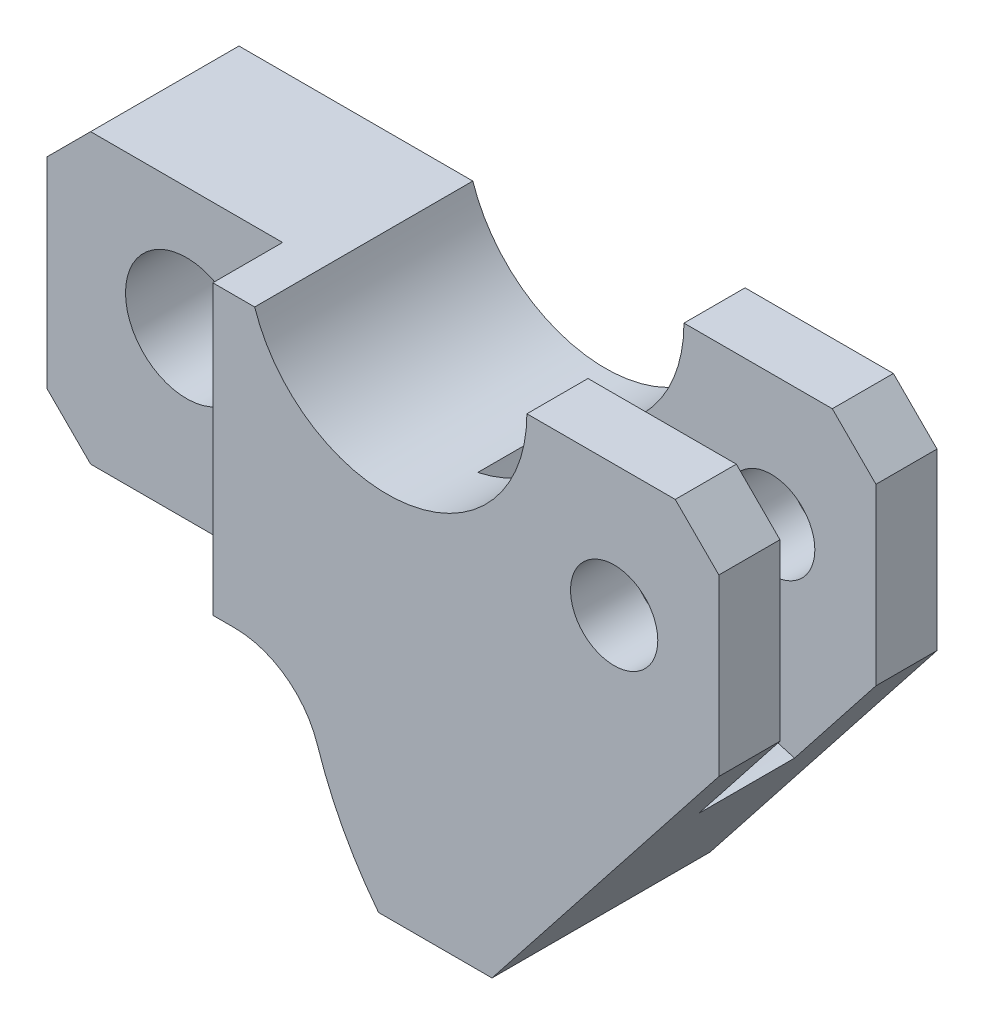
ISO-10303-21;
HEADER;
FILE_DESCRIPTION(('STEP AP214'),'2;1');
FILE_NAME('part.step','',(''),(''),'','','');
FILE_SCHEMA(('AUTOMOTIVE_DESIGN { 1 0 10303 214 1 1 1 1 }'));
ENDSEC;
DATA;
#1=APPLICATION_CONTEXT('core data for automotive mechanical design processes');
#2=APPLICATION_PROTOCOL_DEFINITION('international standard','automotive_design',2000,#1);
#3=PRODUCT_CONTEXT('',#1,'mechanical');
#4=PRODUCT('Part','Part','',(#3));
#5=PRODUCT_RELATED_PRODUCT_CATEGORY('part','',(#4));
#6=PRODUCT_DEFINITION_FORMATION('','',#4);
#7=PRODUCT_DEFINITION_CONTEXT('part definition',#1,'design');
#8=PRODUCT_DEFINITION('design','',#6,#7);
#9=PRODUCT_DEFINITION_SHAPE('','',#8);
#10=(LENGTH_UNIT() NAMED_UNIT(*) SI_UNIT(.MILLI.,.METRE.));
#11=(NAMED_UNIT(*) PLANE_ANGLE_UNIT() SI_UNIT($,.RADIAN.));
#12=(NAMED_UNIT(*) SI_UNIT($,.STERADIAN.) SOLID_ANGLE_UNIT());
#13=UNCERTAINTY_MEASURE_WITH_UNIT(LENGTH_MEASURE(1.E-05),#10,'distance_accuracy_value','');
#14=(GEOMETRIC_REPRESENTATION_CONTEXT(3) GLOBAL_UNCERTAINTY_ASSIGNED_CONTEXT((#13)) GLOBAL_UNIT_ASSIGNED_CONTEXT((#10,
#11,#12)) REPRESENTATION_CONTEXT('',''));
#15=CARTESIAN_POINT('',(0.,0.,0.));
#16=DIRECTION('',(0.,0.,1.));
#17=DIRECTION('',(1.,0.,0.));
#18=AXIS2_PLACEMENT_3D('',#15,#16,#17);
#19=CARTESIAN_POINT('',(0.,-3.84,12.5));
#20=DIRECTION('',(0.,0.,-1.));
#21=DIRECTION('',(-1.,0.,0.));
#22=AXIS2_PLACEMENT_3D('',#19,#20,#21);
#23=CYLINDRICAL_SURFACE('',#22,16.);
#24=CARTESIAN_POINT('',(0.,-3.84,-5.5));
#25=DIRECTION('',(0.,0.,1.));
#26=DIRECTION('',(1.,0.,0.));
#27=AXIS2_PLACEMENT_3D('',#24,#25,#26);
#28=CIRCLE('',#27,16.);
#29=CARTESIAN_POINT('',(16.,-3.84,-5.5));
#30=VERTEX_POINT('',#29);
#31=CARTESIAN_POINT('',(3.3684210526316,-19.4814110492688,-5.5));
#32=VERTEX_POINT('',#31);
#33=EDGE_CURVE('E222',#30,#32,#28,.F.);
#34=ORIENTED_EDGE('',*,*,#33,.F.);
#35=DIRECTION('',(0.,0.,-1.));
#36=VECTOR('',#35,1.);
#37=CARTESIAN_POINT('',(16.,-3.84,12.5));
#38=LINE('',#37,#36);
#39=CARTESIAN_POINT('',(16.,-3.84,-12.5));
#40=VERTEX_POINT('',#39);
#41=EDGE_CURVE('E277',#30,#40,#38,.T.);
#42=ORIENTED_EDGE('',*,*,#41,.T.);
#43=CARTESIAN_POINT('',(0.,-3.84,-12.5));
#44=DIRECTION('',(0.,0.,-1.));
#45=DIRECTION('',(1.,0.,0.));
#46=AXIS2_PLACEMENT_3D('',#43,#44,#45);
#47=CIRCLE('',#46,16.);
#48=CARTESIAN_POINT('',(-15.1986841535706,-8.84,-12.5));
#49=VERTEX_POINT('',#48);
#50=EDGE_CURVE('E251',#40,#49,#47,.T.);
#51=ORIENTED_EDGE('',*,*,#50,.T.);
#52=DIRECTION('',(0.,0.,-1.));
#53=VECTOR('',#52,1.);
#54=CARTESIAN_POINT('',(-15.1986841535706,-8.84,12.5));
#55=LINE('',#54,#53);
#56=CARTESIAN_POINT('',(-15.1986841535706,-8.84,12.5));
#57=VERTEX_POINT('',#56);
#58=EDGE_CURVE('E318',#57,#49,#55,.T.);
#59=ORIENTED_EDGE('',*,*,#58,.F.);
#60=CARTESIAN_POINT('',(0.,-3.84,12.5));
#61=DIRECTION('',(0.,0.,-1.));
#62=DIRECTION('',(1.,0.,0.));
#63=AXIS2_PLACEMENT_3D('',#60,#61,#62);
#64=CIRCLE('',#63,16.);
#65=CARTESIAN_POINT('',(16.,-3.84,12.5));
#66=VERTEX_POINT('',#65);
#67=EDGE_CURVE('E255',#66,#57,#64,.T.);
#68=ORIENTED_EDGE('',*,*,#67,.F.);
#69=CARTESIAN_POINT('',(16.,-3.84,5.5));
#70=VERTEX_POINT('',#69);
#71=EDGE_CURVE('E206',#66,#70,#38,.T.);
#72=ORIENTED_EDGE('',*,*,#71,.T.);
#73=CARTESIAN_POINT('',(0.,-3.84,5.5));
#74=DIRECTION('',(0.,0.,1.));
#75=DIRECTION('',(1.,0.,0.));
#76=AXIS2_PLACEMENT_3D('',#73,#74,#75);
#77=CIRCLE('',#76,16.);
#78=CARTESIAN_POINT('',(3.3684210526316,-19.4814110492688,5.5));
#79=VERTEX_POINT('',#78);
#80=EDGE_CURVE('E200',#70,#79,#77,.F.);
#81=ORIENTED_EDGE('',*,*,#80,.T.);
#82=DIRECTION('',(0.,0.,1.));
#83=VECTOR('',#82,1.);
#84=CARTESIAN_POINT('',(3.3684210526316,-19.4814110492688,0.));
#85=LINE('',#84,#83);
#86=EDGE_CURVE('E188',#79,#32,#85,.F.);
#87=ORIENTED_EDGE('',*,*,#86,.T.);
#88=EDGE_LOOP('',(#34,#42,#51,#59,#68,#72,#81,#87));
#89=FACE_BOUND('',#88,.T.);
#90=ADVANCED_FACE('F41',(#89),#23,.F.);
#91=CARTESIAN_POINT('',(38.,-28.84,12.5));
#92=DIRECTION('',(-0.785491672227536,0.618872226603513,0.));
#93=DIRECTION('',(-0.618872226603513,-0.785491672227536,0.));
#94=AXIS2_PLACEMENT_3D('',#91,#92,#93);
#95=PLANE('',#94);
#96=DIRECTION('',(0.618872226603513,0.785491672227536,0.));
#97=VECTOR('',#96,1.);
#98=CARTESIAN_POINT('',(38.,-28.84,-5.5));
#99=LINE('',#98,#97);
#100=CARTESIAN_POINT('',(28.6733537111755,-40.677666443508,-5.5));
#101=VERTEX_POINT('',#100);
#102=CARTESIAN_POINT('',(38.,-28.84,-5.5));
#103=VERTEX_POINT('',#102);
#104=EDGE_CURVE('E218',#101,#103,#99,.T.);
#105=ORIENTED_EDGE('',*,*,#104,.F.);
#106=DIRECTION('',(0.,0.,1.));
#107=VECTOR('',#106,1.);
#108=CARTESIAN_POINT('',(28.6733537111755,-40.677666443508,-5.5));
#109=LINE('',#108,#107);
#110=CARTESIAN_POINT('',(28.6733537111755,-40.677666443508,5.5));
#111=VERTEX_POINT('',#110);
#112=EDGE_CURVE('E11',#101,#111,#109,.T.);
#113=ORIENTED_EDGE('',*,*,#112,.T.);
#114=DIRECTION('',(0.618872226603513,0.785491672227536,0.));
#115=VECTOR('',#114,1.);
#116=CARTESIAN_POINT('',(38.,-28.84,5.5));
#117=LINE('',#116,#115);
#118=CARTESIAN_POINT('',(38.,-28.84,5.5));
#119=VERTEX_POINT('',#118);
#120=EDGE_CURVE('E203',#111,#119,#117,.T.);
#121=ORIENTED_EDGE('',*,*,#120,.T.);
#122=DIRECTION('',(0.,0.,-1.));
#123=VECTOR('',#122,1.);
#124=CARTESIAN_POINT('',(38.,-28.84,12.5));
#125=LINE('',#124,#123);
#126=CARTESIAN_POINT('',(38.,-28.84,12.5));
#127=VERTEX_POINT('',#126);
#128=EDGE_CURVE('E305',#127,#119,#125,.T.);
#129=ORIENTED_EDGE('',*,*,#128,.F.);
#130=DIRECTION('',(0.618872226603513,0.785491672227535,0.));
#131=VECTOR('',#130,1.);
#132=CARTESIAN_POINT('',(38.,-28.84,12.5));
#133=LINE('',#132,#131);
#134=CARTESIAN_POINT('',(12.,-61.84,12.5));
#135=VERTEX_POINT('',#134);
#136=EDGE_CURVE('E267',#135,#127,#133,.T.);
#137=ORIENTED_EDGE('',*,*,#136,.F.);
#138=DIRECTION('',(0.,0.,-1.));
#139=VECTOR('',#138,1.);
#140=CARTESIAN_POINT('',(12.,-61.84,12.5));
#141=LINE('',#140,#139);
#142=CARTESIAN_POINT('',(12.,-61.84,-12.5));
#143=VERTEX_POINT('',#142);
#144=EDGE_CURVE('E308',#135,#143,#141,.T.);
#145=ORIENTED_EDGE('',*,*,#144,.T.);
#146=DIRECTION('',(0.618872226603513,0.785491672227535,0.));
#147=VECTOR('',#146,1.);
#148=CARTESIAN_POINT('',(38.,-28.84,-12.5));
#149=LINE('',#148,#147);
#150=CARTESIAN_POINT('',(38.,-28.84,-12.5));
#151=VERTEX_POINT('',#150);
#152=EDGE_CURVE('E291',#143,#151,#149,.T.);
#153=ORIENTED_EDGE('',*,*,#152,.T.);
#154=EDGE_CURVE('E301',#103,#151,#125,.T.);
#155=ORIENTED_EDGE('',*,*,#154,.F.);
#156=EDGE_LOOP('',(#105,#113,#121,#129,#137,#145,#153,#155));
#157=FACE_BOUND('',#156,.T.);
#158=ADVANCED_FACE('F392',(#157),#95,.F.);
#159=CARTESIAN_POINT('',(38.,-3.84,12.5));
#160=DIRECTION('',(-1.,0.,0.));
#161=DIRECTION('',(0.,-1.,0.));
#162=AXIS2_PLACEMENT_3D('',#159,#160,#161);
#163=PLANE('',#162);
#164=DIRECTION('',(0.,1.,0.));
#165=VECTOR('',#164,1.);
#166=CARTESIAN_POINT('',(38.,-3.84,-5.5));
#167=LINE('',#166,#165);
#168=CARTESIAN_POINT('',(38.,-8.84000000000001,-5.5));
#169=VERTEX_POINT('',#168);
#170=EDGE_CURVE('E220',#103,#169,#167,.T.);
#171=ORIENTED_EDGE('',*,*,#170,.F.);
#172=ORIENTED_EDGE('',*,*,#154,.T.);
#173=DIRECTION('',(0.,1.,0.));
#174=VECTOR('',#173,1.);
#175=CARTESIAN_POINT('',(38.,-3.84,-12.5));
#176=LINE('',#175,#174);
#177=CARTESIAN_POINT('',(38.,-8.84000000000001,-12.5));
#178=VERTEX_POINT('',#177);
#179=EDGE_CURVE('E298',#151,#178,#176,.T.);
#180=ORIENTED_EDGE('',*,*,#179,.T.);
#181=DIRECTION('',(0.,0.,1.));
#182=VECTOR('',#181,1.);
#183=CARTESIAN_POINT('',(38.,-8.84000000000001,12.5));
#184=LINE('',#183,#182);
#185=EDGE_CURVE('E343',#178,#169,#184,.T.);
#186=ORIENTED_EDGE('',*,*,#185,.T.);
#187=EDGE_LOOP('',(#171,#172,#180,#186));
#188=FACE_BOUND('',#187,.T.);
#189=ADVANCED_FACE('F357',(#188),#163,.F.);
#190=CARTESIAN_POINT('',(16.,-3.84,12.5));
#191=DIRECTION('',(0.,-1.,0.));
#192=DIRECTION('',(1.,0.,0.));
#193=AXIS2_PLACEMENT_3D('',#190,#191,#192);
#194=PLANE('',#193);
#195=DIRECTION('',(-1.,0.,0.));
#196=VECTOR('',#195,1.);
#197=CARTESIAN_POINT('',(16.,-3.84,-5.5));
#198=LINE('',#197,#196);
#199=CARTESIAN_POINT('',(33.,-3.84,-5.5));
#200=VERTEX_POINT('',#199);
#201=EDGE_CURVE('E209',#200,#30,#198,.T.);
#202=ORIENTED_EDGE('',*,*,#201,.F.);
#203=DIRECTION('',(0.,0.,-1.));
#204=VECTOR('',#203,1.);
#205=CARTESIAN_POINT('',(33.,-3.84,12.5));
#206=LINE('',#205,#204);
#207=CARTESIAN_POINT('',(33.,-3.84,-12.5));
#208=VERTEX_POINT('',#207);
#209=EDGE_CURVE('E337',#200,#208,#206,.T.);
#210=ORIENTED_EDGE('',*,*,#209,.T.);
#211=DIRECTION('',(-1.,0.,0.));
#212=VECTOR('',#211,1.);
#213=CARTESIAN_POINT('',(16.,-3.84,-12.5));
#214=LINE('',#213,#212);
#215=EDGE_CURVE('E256',#208,#40,#214,.T.);
#216=ORIENTED_EDGE('',*,*,#215,.T.);
#217=ORIENTED_EDGE('',*,*,#41,.F.);
#218=EDGE_LOOP('',(#202,#210,#216,#217));
#219=FACE_BOUND('',#218,.T.);
#220=ADVANCED_FACE('F373',(#219),#194,.F.);
#221=CARTESIAN_POINT('',(26.,-18.84,12.5));
#222=DIRECTION('',(0.,0.,-1.));
#223=DIRECTION('',(-1.,0.,0.));
#224=AXIS2_PLACEMENT_3D('',#221,#222,#223);
#225=CYLINDRICAL_SURFACE('',#224,5.);
#226=CARTESIAN_POINT('',(26.,-18.84,-12.5));
#227=DIRECTION('',(0.,0.,1.));
#228=DIRECTION('',(1.,0.,0.));
#229=AXIS2_PLACEMENT_3D('',#226,#227,#228);
#230=CIRCLE('',#229,5.);
#231=CARTESIAN_POINT('',(31.,-18.84,-12.5));
#232=VERTEX_POINT('',#231);
#233=EDGE_CURVE('E242',#232,#232,#230,.T.);
#234=ORIENTED_EDGE('',*,*,#233,.F.);
#235=EDGE_LOOP('',(#234));
#236=FACE_BOUND('',#235,.T.);
#237=CARTESIAN_POINT('',(26.,-18.84,-5.5));
#238=DIRECTION('',(0.,0.,1.));
#239=DIRECTION('',(1.,0.,0.));
#240=AXIS2_PLACEMENT_3D('',#237,#238,#239);
#241=CIRCLE('',#240,5.);
#242=CARTESIAN_POINT('',(31.,-18.84,-5.5));
#243=VERTEX_POINT('',#242);
#244=EDGE_CURVE('E198',#243,#243,#241,.T.);
#245=ORIENTED_EDGE('',*,*,#244,.T.);
#246=EDGE_LOOP('',(#245));
#247=FACE_BOUND('',#246,.T.);
#248=ADVANCED_FACE('F448',(#236,#247),#225,.F.);
#249=CARTESIAN_POINT('',(33.,-3.84,12.5));
#250=DIRECTION('',(-0.707106781186548,-0.707106781186546,0.));
#251=DIRECTION('',(0.,0.,-1.));
#252=AXIS2_PLACEMENT_3D('',#249,#250,#251);
#253=PLANE('',#252);
#254=ORIENTED_EDGE('',*,*,#209,.F.);
#255=DIRECTION('',(-0.707106781186547,0.707106781186549,0.));
#256=VECTOR('',#255,1.);
#257=CARTESIAN_POINT('',(33.,-3.84,-5.5));
#258=LINE('',#257,#256);
#259=EDGE_CURVE('E49',#200,#169,#258,.F.);
#260=ORIENTED_EDGE('',*,*,#259,.T.);
#261=ORIENTED_EDGE('',*,*,#185,.F.);
#262=DIRECTION('',(-0.707106781186547,0.707106781186549,0.));
#263=VECTOR('',#262,1.);
#264=CARTESIAN_POINT('',(33.,-3.84,-12.5));
#265=LINE('',#264,#263);
#266=EDGE_CURVE('E326',#208,#178,#265,.F.);
#267=ORIENTED_EDGE('',*,*,#266,.F.);
#268=EDGE_LOOP('',(#254,#260,#261,#267));
#269=FACE_BOUND('',#268,.T.);
#270=ADVANCED_FACE('F352',(#269),#253,.F.);
#271=CARTESIAN_POINT('',(0.,-3.84,12.5));
#272=DIRECTION('',(0.,0.,1.));
#273=DIRECTION('',(1.,0.,0.));
#274=AXIS2_PLACEMENT_3D('',#271,#272,#273);
#275=PLANE('',#274);
#276=DIRECTION('',(0.,1.,0.));
#277=VECTOR('',#276,1.);
#278=CARTESIAN_POINT('',(-20.,-8.84,12.5));
#279=LINE('',#278,#277);
#280=CARTESIAN_POINT('',(-20.,-41.84,12.5));
#281=VERTEX_POINT('',#280);
#282=CARTESIAN_POINT('',(-20.,-8.84,12.5));
#283=VERTEX_POINT('',#282);
#284=EDGE_CURVE('E192',#281,#283,#279,.T.);
#285=ORIENTED_EDGE('',*,*,#284,.F.);
#286=DIRECTION('',(1.,0.,0.));
#287=VECTOR('',#286,1.);
#288=CARTESIAN_POINT('',(-47.,-41.84,12.5));
#289=LINE('',#288,#287);
#290=CARTESIAN_POINT('',(-17.5042005852112,-41.84,12.5));
#291=VERTEX_POINT('',#290);
#292=EDGE_CURVE('E261',#281,#291,#289,.T.);
#293=ORIENTED_EDGE('',*,*,#292,.T.);
#294=CARTESIAN_POINT('',(-17.5042005852112,-51.84,12.5));
#295=DIRECTION('',(0.,0.,-1.));
#296=DIRECTION('',(1.,0.,0.));
#297=AXIS2_PLACEMENT_3D('',#294,#295,#296);
#298=CIRCLE('',#297,10.);
#299=CARTESIAN_POINT('',(-8.00180676846029,-48.7247934656955,12.5));
#300=VERTEX_POINT('',#299);
#301=EDGE_CURVE('E263',#291,#300,#298,.T.);
#302=ORIENTED_EDGE('',*,*,#301,.T.);
#303=CARTESIAN_POINT('',(32.8971117805512,-35.3167427400696,12.5));
#304=DIRECTION('',(0.,0.,1.));
#305=DIRECTION('',(1.,0.,0.));
#306=AXIS2_PLACEMENT_3D('',#303,#304,#305);
#307=CIRCLE('',#306,43.0406477964683);
#308=CARTESIAN_POINT('',(-0.999999999999987,-61.84,12.5));
#309=VERTEX_POINT('',#308);
#310=EDGE_CURVE('E264',#300,#309,#307,.T.);
#311=ORIENTED_EDGE('',*,*,#310,.T.);
#312=DIRECTION('',(1.,0.,0.));
#313=VECTOR('',#312,1.);
#314=CARTESIAN_POINT('',(12.,-61.84,12.5));
#315=LINE('',#314,#313);
#316=EDGE_CURVE('E270',#309,#135,#315,.T.);
#317=ORIENTED_EDGE('',*,*,#316,.T.);
#318=ORIENTED_EDGE('',*,*,#136,.T.);
#319=DIRECTION('',(0.,1.,0.));
#320=VECTOR('',#319,1.);
#321=CARTESIAN_POINT('',(38.,-3.84,12.5));
#322=LINE('',#321,#320);
#323=CARTESIAN_POINT('',(38.,-8.84000000000001,12.5));
#324=VERTEX_POINT('',#323);
#325=EDGE_CURVE('E271',#127,#324,#322,.T.);
#326=ORIENTED_EDGE('',*,*,#325,.T.);
#327=DIRECTION('',(0.707106781186547,-0.707106781186549,0.));
#328=VECTOR('',#327,1.);
#329=CARTESIAN_POINT('',(16.5000000000001,12.66,12.5));
#330=LINE('',#329,#328);
#331=CARTESIAN_POINT('',(33.,-3.84,12.5));
#332=VERTEX_POINT('',#331);
#333=EDGE_CURVE('E333',#324,#332,#330,.F.);
#334=ORIENTED_EDGE('',*,*,#333,.T.);
#335=DIRECTION('',(-1.,0.,0.));
#336=VECTOR('',#335,1.);
#337=CARTESIAN_POINT('',(16.,-3.84,12.5));
#338=LINE('',#337,#336);
#339=EDGE_CURVE('E273',#332,#66,#338,.T.);
#340=ORIENTED_EDGE('',*,*,#339,.T.);
#341=ORIENTED_EDGE('',*,*,#67,.T.);
#342=DIRECTION('',(-1.,0.,0.));
#343=VECTOR('',#342,1.);
#344=CARTESIAN_POINT('',(-15.1986841535706,-8.84,12.5));
#345=LINE('',#344,#343);
#346=EDGE_CURVE('E260',#57,#283,#345,.T.);
#347=ORIENTED_EDGE('',*,*,#346,.T.);
#348=EDGE_LOOP('',(#285,#293,#302,#311,#317,#318,#326,#334,#340,#341,#347));
#349=FACE_BOUND('',#348,.T.);
#350=CARTESIAN_POINT('',(26.,-18.84,12.5));
#351=DIRECTION('',(0.,0.,1.));
#352=DIRECTION('',(1.,0.,0.));
#353=AXIS2_PLACEMENT_3D('',#350,#351,#352);
#354=CIRCLE('',#353,5.);
#355=CARTESIAN_POINT('',(31.,-18.84,12.5));
#356=VERTEX_POINT('',#355);
#357=EDGE_CURVE('E244',#356,#356,#354,.T.);
#358=ORIENTED_EDGE('',*,*,#357,.F.);
#359=EDGE_LOOP('',(#358));
#360=FACE_BOUND('',#359,.T.);
#361=ADVANCED_FACE('F385',(#349,#360),#275,.T.);
#362=CARTESIAN_POINT('',(0.,-3.84,-12.5));
#363=DIRECTION('',(0.,0.,1.));
#364=DIRECTION('',(1.,0.,0.));
#365=AXIS2_PLACEMENT_3D('',#362,#363,#364);
#366=PLANE('',#365);
#367=DIRECTION('',(0.,-1.,0.));
#368=VECTOR('',#367,1.);
#369=CARTESIAN_POINT('',(-47.,-8.84,-12.5));
#370=LINE('',#369,#368);
#371=CARTESIAN_POINT('',(-47.,-13.84,-12.5));
#372=VERTEX_POINT('',#371);
#373=CARTESIAN_POINT('',(-47.,-36.84,-12.5));
#374=VERTEX_POINT('',#373);
#375=EDGE_CURVE('E285',#372,#374,#370,.T.);
#376=ORIENTED_EDGE('',*,*,#375,.F.);
#377=DIRECTION('',(-0.707106781186548,-0.707106781186547,0.));
#378=VECTOR('',#377,1.);
#379=CARTESIAN_POINT('',(-47.,-13.84,-12.5));
#380=LINE('',#379,#378);
#381=CARTESIAN_POINT('',(-42.,-8.84,-12.5));
#382=VERTEX_POINT('',#381);
#383=EDGE_CURVE('E329',#372,#382,#380,.F.);
#384=ORIENTED_EDGE('',*,*,#383,.T.);
#385=DIRECTION('',(-1.,0.,0.));
#386=VECTOR('',#385,1.);
#387=CARTESIAN_POINT('',(-15.1986841535706,-8.84,-12.5));
#388=LINE('',#387,#386);
#389=EDGE_CURVE('E276',#49,#382,#388,.T.);
#390=ORIENTED_EDGE('',*,*,#389,.F.);
#391=ORIENTED_EDGE('',*,*,#50,.F.);
#392=ORIENTED_EDGE('',*,*,#215,.F.);
#393=ORIENTED_EDGE('',*,*,#266,.T.);
#394=ORIENTED_EDGE('',*,*,#179,.F.);
#395=ORIENTED_EDGE('',*,*,#152,.F.);
#396=DIRECTION('',(1.,0.,0.));
#397=VECTOR('',#396,1.);
#398=CARTESIAN_POINT('',(12.,-61.84,-12.5));
#399=LINE('',#398,#397);
#400=CARTESIAN_POINT('',(-0.999999999999987,-61.84,-12.5));
#401=VERTEX_POINT('',#400);
#402=EDGE_CURVE('E292',#401,#143,#399,.T.);
#403=ORIENTED_EDGE('',*,*,#402,.F.);
#404=CARTESIAN_POINT('',(32.8971117805512,-35.3167427400696,-12.5));
#405=DIRECTION('',(0.,0.,1.));
#406=DIRECTION('',(1.,0.,0.));
#407=AXIS2_PLACEMENT_3D('',#404,#405,#406);
#408=CIRCLE('',#407,43.0406477964683);
#409=CARTESIAN_POINT('',(-8.00180676846029,-48.7247934656955,-12.5));
#410=VERTEX_POINT('',#409);
#411=EDGE_CURVE('E288',#410,#401,#408,.T.);
#412=ORIENTED_EDGE('',*,*,#411,.F.);
#413=CARTESIAN_POINT('',(-17.5042005852112,-51.84,-12.5));
#414=DIRECTION('',(0.,0.,-1.));
#415=DIRECTION('',(1.,0.,0.));
#416=AXIS2_PLACEMENT_3D('',#413,#414,#415);
#417=CIRCLE('',#416,10.);
#418=CARTESIAN_POINT('',(-17.5042005852112,-41.84,-12.5));
#419=VERTEX_POINT('',#418);
#420=EDGE_CURVE('E286',#419,#410,#417,.T.);
#421=ORIENTED_EDGE('',*,*,#420,.F.);
#422=DIRECTION('',(1.,0.,0.));
#423=VECTOR('',#422,1.);
#424=CARTESIAN_POINT('',(-47.,-41.84,-12.5));
#425=LINE('',#424,#423);
#426=CARTESIAN_POINT('',(-42.,-41.84,-12.5));
#427=VERTEX_POINT('',#426);
#428=EDGE_CURVE('E284',#427,#419,#425,.T.);
#429=ORIENTED_EDGE('',*,*,#428,.F.);
#430=DIRECTION('',(0.707106781186546,-0.707106781186549,0.));
#431=VECTOR('',#430,1.);
#432=CARTESIAN_POINT('',(-42.,-41.84,-12.5));
#433=LINE('',#432,#431);
#434=EDGE_CURVE('E327',#427,#374,#433,.F.);
#435=ORIENTED_EDGE('',*,*,#434,.T.);
#436=EDGE_LOOP('',(#376,#384,#390,#391,#392,#393,#394,#395,#403,#412,#421,#429,#435));
#437=FACE_BOUND('',#436,.T.);
#438=CARTESIAN_POINT('',(-31.,-22.84,-12.5));
#439=DIRECTION('',(0.,0.,1.));
#440=DIRECTION('',(1.,0.,0.));
#441=AXIS2_PLACEMENT_3D('',#438,#439,#440);
#442=CIRCLE('',#441,7.);
#443=CARTESIAN_POINT('',(-24.,-22.84,-12.5));
#444=VERTEX_POINT('',#443);
#445=EDGE_CURVE('E250',#444,#444,#442,.T.);
#446=ORIENTED_EDGE('',*,*,#445,.T.);
#447=EDGE_LOOP('',(#446));
#448=FACE_BOUND('',#447,.T.);
#449=ORIENTED_EDGE('',*,*,#233,.T.);
#450=EDGE_LOOP('',(#449));
#451=FACE_BOUND('',#450,.T.);
#452=ADVANCED_FACE('F368',(#437,#448,#451),#366,.F.);
#453=CARTESIAN_POINT('',(-15.1986841535706,-8.84,12.5));
#454=DIRECTION('',(0.,-1.,0.));
#455=DIRECTION('',(1.,0.,0.));
#456=AXIS2_PLACEMENT_3D('',#453,#454,#455);
#457=PLANE('',#456);
#458=DIRECTION('',(-1.,0.,0.));
#459=VECTOR('',#458,1.);
#460=CARTESIAN_POINT('',(-47.,-8.84,4.5));
#461=LINE('',#460,#459);
#462=CARTESIAN_POINT('',(-20.,-8.84,4.5));
#463=VERTEX_POINT('',#462);
#464=CARTESIAN_POINT('',(-42.,-8.84,4.5));
#465=VERTEX_POINT('',#464);
#466=EDGE_CURVE('E229',#463,#465,#461,.T.);
#467=ORIENTED_EDGE('',*,*,#466,.F.);
#468=DIRECTION('',(0.,0.,1.));
#469=VECTOR('',#468,1.);
#470=CARTESIAN_POINT('',(-20.,-8.84,4.5));
#471=LINE('',#470,#469);
#472=EDGE_CURVE('E232',#463,#283,#471,.T.);
#473=ORIENTED_EDGE('',*,*,#472,.T.);
#474=ORIENTED_EDGE('',*,*,#346,.F.);
#475=ORIENTED_EDGE('',*,*,#58,.T.);
#476=ORIENTED_EDGE('',*,*,#389,.T.);
#477=DIRECTION('',(0.,0.,1.));
#478=VECTOR('',#477,1.);
#479=CARTESIAN_POINT('',(-42.,-8.84,12.5));
#480=LINE('',#479,#478);
#481=EDGE_CURVE('E335',#382,#465,#480,.T.);
#482=ORIENTED_EDGE('',*,*,#481,.T.);
#483=EDGE_LOOP('',(#467,#473,#474,#475,#476,#482));
#484=FACE_BOUND('',#483,.T.);
#485=ADVANCED_FACE('F378',(#484),#457,.F.);
#486=CARTESIAN_POINT('',(-47.,-8.84,12.5));
#487=DIRECTION('',(1.,0.,0.));
#488=DIRECTION('',(0.,0.,-1.));
#489=AXIS2_PLACEMENT_3D('',#486,#487,#488);
#490=PLANE('',#489);
#491=DIRECTION('',(0.,0.,1.));
#492=VECTOR('',#491,1.);
#493=CARTESIAN_POINT('',(-47.,-36.84,12.5));
#494=LINE('',#493,#492);
#495=CARTESIAN_POINT('',(-47.,-36.84,4.5));
#496=VERTEX_POINT('',#495);
#497=EDGE_CURVE('E321',#374,#496,#494,.T.);
#498=ORIENTED_EDGE('',*,*,#497,.T.);
#499=DIRECTION('',(0.,-1.,0.));
#500=VECTOR('',#499,1.);
#501=CARTESIAN_POINT('',(-47.,-8.84,4.5));
#502=LINE('',#501,#500);
#503=CARTESIAN_POINT('',(-47.,-13.84,4.5));
#504=VERTEX_POINT('',#503);
#505=EDGE_CURVE('E64',#504,#496,#502,.T.);
#506=ORIENTED_EDGE('',*,*,#505,.F.);
#507=DIRECTION('',(0.,0.,-1.));
#508=VECTOR('',#507,1.);
#509=CARTESIAN_POINT('',(-47.,-13.84,12.5));
#510=LINE('',#509,#508);
#511=EDGE_CURVE('E322',#504,#372,#510,.T.);
#512=ORIENTED_EDGE('',*,*,#511,.T.);
#513=ORIENTED_EDGE('',*,*,#375,.T.);
#514=EDGE_LOOP('',(#498,#506,#512,#513));
#515=FACE_BOUND('',#514,.T.);
#516=ADVANCED_FACE('F421',(#515),#490,.F.);
#517=CARTESIAN_POINT('',(-47.,-41.84,12.5));
#518=DIRECTION('',(0.,1.,0.));
#519=DIRECTION('',(0.,0.,1.));
#520=AXIS2_PLACEMENT_3D('',#517,#518,#519);
#521=PLANE('',#520);
#522=ORIENTED_EDGE('',*,*,#292,.F.);
#523=DIRECTION('',(0.,0.,1.));
#524=VECTOR('',#523,1.);
#525=CARTESIAN_POINT('',(-20.,-41.84,4.5));
#526=LINE('',#525,#524);
#527=CARTESIAN_POINT('',(-20.,-41.84,4.5));
#528=VERTEX_POINT('',#527);
#529=EDGE_CURVE('E235',#528,#281,#526,.T.);
#530=ORIENTED_EDGE('',*,*,#529,.F.);
#531=DIRECTION('',(1.,0.,0.));
#532=VECTOR('',#531,1.);
#533=CARTESIAN_POINT('',(-47.,-41.84,4.5));
#534=LINE('',#533,#532);
#535=CARTESIAN_POINT('',(-42.,-41.84,4.5));
#536=VERTEX_POINT('',#535);
#537=EDGE_CURVE('E223',#536,#528,#534,.T.);
#538=ORIENTED_EDGE('',*,*,#537,.F.);
#539=DIRECTION('',(0.,0.,-1.));
#540=VECTOR('',#539,1.);
#541=CARTESIAN_POINT('',(-42.,-41.84,12.5));
#542=LINE('',#541,#540);
#543=EDGE_CURVE('E340',#536,#427,#542,.T.);
#544=ORIENTED_EDGE('',*,*,#543,.T.);
#545=ORIENTED_EDGE('',*,*,#428,.T.);
#546=DIRECTION('',(0.,0.,-1.));
#547=VECTOR('',#546,1.);
#548=CARTESIAN_POINT('',(-17.5042005852112,-41.84,12.5));
#549=LINE('',#548,#547);
#550=EDGE_CURVE('E312',#291,#419,#549,.T.);
#551=ORIENTED_EDGE('',*,*,#550,.F.);
#552=EDGE_LOOP('',(#522,#530,#538,#544,#545,#551));
#553=FACE_BOUND('',#552,.T.);
#554=ADVANCED_FACE('F412',(#553),#521,.F.);
#555=CARTESIAN_POINT('',(-17.5042005852112,-51.84,12.5));
#556=DIRECTION('',(0.,0.,-1.));
#557=DIRECTION('',(-1.,0.,0.));
#558=AXIS2_PLACEMENT_3D('',#555,#556,#557);
#559=CYLINDRICAL_SURFACE('',#558,10.);
#560=ORIENTED_EDGE('',*,*,#420,.T.);
#561=DIRECTION('',(0.,0.,-1.));
#562=VECTOR('',#561,1.);
#563=CARTESIAN_POINT('',(-8.00180676846029,-48.7247934656955,12.5));
#564=LINE('',#563,#562);
#565=EDGE_CURVE('E315',#300,#410,#564,.T.);
#566=ORIENTED_EDGE('',*,*,#565,.F.);
#567=ORIENTED_EDGE('',*,*,#301,.F.);
#568=ORIENTED_EDGE('',*,*,#550,.T.);
#569=EDGE_LOOP('',(#560,#566,#567,#568));
#570=FACE_BOUND('',#569,.T.);
#571=ADVANCED_FACE('F414',(#570),#559,.F.);
#572=CARTESIAN_POINT('',(32.8971117805512,-35.3167427400696,12.5));
#573=DIRECTION('',(0.,0.,-1.));
#574=DIRECTION('',(-1.,0.,0.));
#575=AXIS2_PLACEMENT_3D('',#572,#573,#574);
#576=CYLINDRICAL_SURFACE('',#575,43.0406477964683);
#577=ORIENTED_EDGE('',*,*,#411,.T.);
#578=DIRECTION('',(0.,0.,-1.));
#579=VECTOR('',#578,1.);
#580=CARTESIAN_POINT('',(-0.999999999999987,-61.84,12.5));
#581=LINE('',#580,#579);
#582=EDGE_CURVE('E310',#309,#401,#581,.T.);
#583=ORIENTED_EDGE('',*,*,#582,.F.);
#584=ORIENTED_EDGE('',*,*,#310,.F.);
#585=ORIENTED_EDGE('',*,*,#565,.T.);
#586=EDGE_LOOP('',(#577,#583,#584,#585));
#587=FACE_BOUND('',#586,.T.);
#588=ADVANCED_FACE('F408',(#587),#576,.T.);
#589=CARTESIAN_POINT('',(12.,-61.84,12.5));
#590=DIRECTION('',(0.,1.,0.));
#591=DIRECTION('',(-1.,0.,0.));
#592=AXIS2_PLACEMENT_3D('',#589,#590,#591);
#593=PLANE('',#592);
#594=ORIENTED_EDGE('',*,*,#402,.T.);
#595=ORIENTED_EDGE('',*,*,#144,.F.);
#596=ORIENTED_EDGE('',*,*,#316,.F.);
#597=ORIENTED_EDGE('',*,*,#582,.T.);
#598=EDGE_LOOP('',(#594,#595,#596,#597));
#599=FACE_BOUND('',#598,.T.);
#600=ADVANCED_FACE('F397',(#599),#593,.F.);
#601=ORIENTED_EDGE('',*,*,#128,.T.);
#602=DIRECTION('',(0.,1.,0.));
#603=VECTOR('',#602,1.);
#604=CARTESIAN_POINT('',(38.,-3.84,5.5));
#605=LINE('',#604,#603);
#606=CARTESIAN_POINT('',(38.,-8.84000000000001,5.5));
#607=VERTEX_POINT('',#606);
#608=EDGE_CURVE('E215',#119,#607,#605,.T.);
#609=ORIENTED_EDGE('',*,*,#608,.T.);
#610=EDGE_CURVE('E345',#607,#324,#184,.T.);
#611=ORIENTED_EDGE('',*,*,#610,.T.);
#612=ORIENTED_EDGE('',*,*,#325,.F.);
#613=EDGE_LOOP('',(#601,#609,#611,#612));
#614=FACE_BOUND('',#613,.T.);
#615=ADVANCED_FACE('F433',(#614),#163,.F.);
#616=CARTESIAN_POINT('',(33.,-3.84,5.5));
#617=VERTEX_POINT('',#616);
#618=EDGE_CURVE('E339',#332,#617,#206,.T.);
#619=ORIENTED_EDGE('',*,*,#618,.T.);
#620=DIRECTION('',(-1.,0.,0.));
#621=VECTOR('',#620,1.);
#622=CARTESIAN_POINT('',(16.,-3.84,5.5));
#623=LINE('',#622,#621);
#624=EDGE_CURVE('E60',#617,#70,#623,.T.);
#625=ORIENTED_EDGE('',*,*,#624,.T.);
#626=ORIENTED_EDGE('',*,*,#71,.F.);
#627=ORIENTED_EDGE('',*,*,#339,.F.);
#628=EDGE_LOOP('',(#619,#625,#626,#627));
#629=FACE_BOUND('',#628,.T.);
#630=ADVANCED_FACE('F389',(#629),#194,.F.);
#631=CARTESIAN_POINT('',(-31.,-22.84,12.5));
#632=DIRECTION('',(0.,0.,-1.));
#633=DIRECTION('',(-1.,0.,0.));
#634=AXIS2_PLACEMENT_3D('',#631,#632,#633);
#635=CYLINDRICAL_SURFACE('',#634,7.);
#636=CARTESIAN_POINT('',(-31.,-22.84,4.5));
#637=DIRECTION('',(0.,0.,-1.));
#638=DIRECTION('',(-1.,0.,0.));
#639=AXIS2_PLACEMENT_3D('',#636,#637,#638);
#640=CIRCLE('',#639,7.);
#641=CARTESIAN_POINT('',(-38.,-22.84,4.5));
#642=VERTEX_POINT('',#641);
#643=EDGE_CURVE('E243',#642,#642,#640,.T.);
#644=ORIENTED_EDGE('',*,*,#643,.F.);
#645=EDGE_LOOP('',(#644));
#646=FACE_BOUND('',#645,.T.);
#647=ORIENTED_EDGE('',*,*,#445,.F.);
#648=EDGE_LOOP('',(#647));
#649=FACE_BOUND('',#648,.T.);
#650=ADVANCED_FACE('F473',(#646,#649),#635,.F.);
#651=CARTESIAN_POINT('',(26.,-18.84,5.5));
#652=DIRECTION('',(0.,0.,1.));
#653=DIRECTION('',(1.,0.,0.));
#654=AXIS2_PLACEMENT_3D('',#651,#652,#653);
#655=CIRCLE('',#654,5.);
#656=CARTESIAN_POINT('',(31.,-18.84,5.5));
#657=VERTEX_POINT('',#656);
#658=EDGE_CURVE('E210',#657,#657,#655,.T.);
#659=ORIENTED_EDGE('',*,*,#658,.F.);
#660=EDGE_LOOP('',(#659));
#661=FACE_BOUND('',#660,.T.);
#662=ORIENTED_EDGE('',*,*,#357,.T.);
#663=EDGE_LOOP('',(#662));
#664=FACE_BOUND('',#663,.T.);
#665=ADVANCED_FACE('F465',(#661,#664),#225,.F.);
#666=CARTESIAN_POINT('',(-47.,-13.84,12.5));
#667=DIRECTION('',(0.707106781186547,-0.707106781186548,0.));
#668=DIRECTION('',(0.,0.,-1.));
#669=AXIS2_PLACEMENT_3D('',#666,#667,#668);
#670=PLANE('',#669);
#671=DIRECTION('',(0.707106781186548,0.707106781186547,0.));
#672=VECTOR('',#671,1.);
#673=CARTESIAN_POINT('',(-47.,-13.84,4.5));
#674=LINE('',#673,#672);
#675=EDGE_CURVE('E236',#465,#504,#674,.F.);
#676=ORIENTED_EDGE('',*,*,#675,.F.);
#677=ORIENTED_EDGE('',*,*,#481,.F.);
#678=ORIENTED_EDGE('',*,*,#383,.F.);
#679=ORIENTED_EDGE('',*,*,#511,.F.);
#680=EDGE_LOOP('',(#676,#677,#678,#679));
#681=FACE_BOUND('',#680,.T.);
#682=ADVANCED_FACE('F441',(#681),#670,.F.);
#683=CARTESIAN_POINT('',(-42.,-41.84,12.5));
#684=DIRECTION('',(0.707106781186549,0.707106781186546,0.));
#685=DIRECTION('',(0.,0.,-1.));
#686=AXIS2_PLACEMENT_3D('',#683,#684,#685);
#687=PLANE('',#686);
#688=DIRECTION('',(-0.707106781186546,0.707106781186549,0.));
#689=VECTOR('',#688,1.);
#690=CARTESIAN_POINT('',(-42.,-41.84,4.5));
#691=LINE('',#690,#689);
#692=EDGE_CURVE('E350',#496,#536,#691,.F.);
#693=ORIENTED_EDGE('',*,*,#692,.F.);
#694=ORIENTED_EDGE('',*,*,#497,.F.);
#695=ORIENTED_EDGE('',*,*,#434,.F.);
#696=ORIENTED_EDGE('',*,*,#543,.F.);
#697=EDGE_LOOP('',(#693,#694,#695,#696));
#698=FACE_BOUND('',#697,.T.);
#699=ADVANCED_FACE('F426',(#698),#687,.F.);
#700=DIRECTION('',(-0.707106781186547,0.707106781186549,0.));
#701=VECTOR('',#700,1.);
#702=CARTESIAN_POINT('',(33.,-3.84,5.5));
#703=LINE('',#702,#701);
#704=EDGE_CURVE('E349',#617,#607,#703,.F.);
#705=ORIENTED_EDGE('',*,*,#704,.F.);
#706=ORIENTED_EDGE('',*,*,#618,.F.);
#707=ORIENTED_EDGE('',*,*,#333,.F.);
#708=ORIENTED_EDGE('',*,*,#610,.F.);
#709=EDGE_LOOP('',(#705,#706,#707,#708));
#710=FACE_BOUND('',#709,.T.);
#711=ADVANCED_FACE('F42',(#710),#253,.F.);
#712=CARTESIAN_POINT('',(-20.,-8.84,4.5));
#713=DIRECTION('',(1.,0.,0.));
#714=DIRECTION('',(0.,1.,0.));
#715=AXIS2_PLACEMENT_3D('',#712,#713,#714);
#716=PLANE('',#715);
#717=ORIENTED_EDGE('',*,*,#284,.T.);
#718=ORIENTED_EDGE('',*,*,#472,.F.);
#719=DIRECTION('',(0.,1.,0.));
#720=VECTOR('',#719,1.);
#721=CARTESIAN_POINT('',(-20.,-8.84,4.5));
#722=LINE('',#721,#720);
#723=EDGE_CURVE('E230',#528,#463,#722,.T.);
#724=ORIENTED_EDGE('',*,*,#723,.F.);
#725=ORIENTED_EDGE('',*,*,#529,.T.);
#726=EDGE_LOOP('',(#717,#718,#724,#725));
#727=FACE_BOUND('',#726,.T.);
#728=ADVANCED_FACE('F429',(#727),#716,.F.);
#729=CARTESIAN_POINT('',(0.,0.,4.5));
#730=DIRECTION('',(0.,0.,-1.));
#731=DIRECTION('',(-1.,0.,0.));
#732=AXIS2_PLACEMENT_3D('',#729,#730,#731);
#733=PLANE('',#732);
#734=ORIENTED_EDGE('',*,*,#643,.T.);
#735=EDGE_LOOP('',(#734));
#736=FACE_BOUND('',#735,.T.);
#737=ORIENTED_EDGE('',*,*,#675,.T.);
#738=ORIENTED_EDGE('',*,*,#505,.T.);
#739=ORIENTED_EDGE('',*,*,#692,.T.);
#740=ORIENTED_EDGE('',*,*,#537,.T.);
#741=ORIENTED_EDGE('',*,*,#723,.T.);
#742=ORIENTED_EDGE('',*,*,#466,.T.);
#743=EDGE_LOOP('',(#737,#738,#739,#740,#741,#742));
#744=FACE_BOUND('',#743,.T.);
#745=ADVANCED_FACE('F430',(#736,#744),#733,.F.);
#746=CARTESIAN_POINT('',(38.,-3.84,-5.5));
#747=DIRECTION('',(0.,0.,1.));
#748=DIRECTION('',(1.,0.,0.));
#749=AXIS2_PLACEMENT_3D('',#746,#747,#748);
#750=CYLINDRICAL_SURFACE('',#749,38.);
#751=CARTESIAN_POINT('',(38.,-3.84,5.5));
#752=DIRECTION('',(0.,0.,1.));
#753=DIRECTION('',(1.,0.,0.));
#754=AXIS2_PLACEMENT_3D('',#751,#752,#753);
#755=CIRCLE('',#754,38.);
#756=EDGE_CURVE('E187',#79,#111,#755,.T.);
#757=ORIENTED_EDGE('',*,*,#756,.T.);
#758=ORIENTED_EDGE('',*,*,#112,.F.);
#759=CARTESIAN_POINT('',(38.,-3.84,-5.5));
#760=DIRECTION('',(0.,0.,1.));
#761=DIRECTION('',(1.,0.,0.));
#762=AXIS2_PLACEMENT_3D('',#759,#760,#761);
#763=CIRCLE('',#762,38.);
#764=EDGE_CURVE('E194',#32,#101,#763,.T.);
#765=ORIENTED_EDGE('',*,*,#764,.F.);
#766=ORIENTED_EDGE('',*,*,#86,.F.);
#767=EDGE_LOOP('',(#757,#758,#765,#766));
#768=FACE_BOUND('',#767,.T.);
#769=ADVANCED_FACE('F186',(#768),#750,.F.);
#770=CARTESIAN_POINT('',(38.,-3.84,-5.5));
#771=DIRECTION('',(0.,0.,1.));
#772=DIRECTION('',(1.,0.,0.));
#773=AXIS2_PLACEMENT_3D('',#770,#771,#772);
#774=PLANE('',#773);
#775=ORIENTED_EDGE('',*,*,#244,.F.);
#776=EDGE_LOOP('',(#775));
#777=FACE_BOUND('',#776,.T.);
#778=ORIENTED_EDGE('',*,*,#33,.T.);
#779=ORIENTED_EDGE('',*,*,#764,.T.);
#780=ORIENTED_EDGE('',*,*,#104,.T.);
#781=ORIENTED_EDGE('',*,*,#170,.T.);
#782=ORIENTED_EDGE('',*,*,#259,.F.);
#783=ORIENTED_EDGE('',*,*,#201,.T.);
#784=EDGE_LOOP('',(#778,#779,#780,#781,#782,#783));
#785=FACE_BOUND('',#784,.T.);
#786=ADVANCED_FACE('F372',(#777,#785),#774,.T.);
#787=CARTESIAN_POINT('',(38.,-3.84,5.5));
#788=DIRECTION('',(0.,0.,1.));
#789=DIRECTION('',(1.,0.,0.));
#790=AXIS2_PLACEMENT_3D('',#787,#788,#789);
#791=PLANE('',#790);
#792=ORIENTED_EDGE('',*,*,#658,.T.);
#793=EDGE_LOOP('',(#792));
#794=FACE_BOUND('',#793,.T.);
#795=ORIENTED_EDGE('',*,*,#624,.F.);
#796=ORIENTED_EDGE('',*,*,#704,.T.);
#797=ORIENTED_EDGE('',*,*,#608,.F.);
#798=ORIENTED_EDGE('',*,*,#120,.F.);
#799=ORIENTED_EDGE('',*,*,#756,.F.);
#800=ORIENTED_EDGE('',*,*,#80,.F.);
#801=EDGE_LOOP('',(#795,#796,#797,#798,#799,#800));
#802=FACE_BOUND('',#801,.T.);
#803=ADVANCED_FACE('F196',(#794,#802),#791,.F.);
#804=CLOSED_SHELL('',(#90,#158,#189,#220,#248,#270,#361,#452,#485,#516,#554,#571,#588,#600,#615,
#630,#650,#665,#682,#699,#711,#728,#745,#769,#786,#803));
#805=MANIFOLD_SOLID_BREP('B2',#804);
#806=ADVANCED_BREP_SHAPE_REPRESENTATION('',(#18,#805),#14);
#807=SHAPE_DEFINITION_REPRESENTATION(#9,#806);
ENDSEC;
END-ISO-10303-21;
